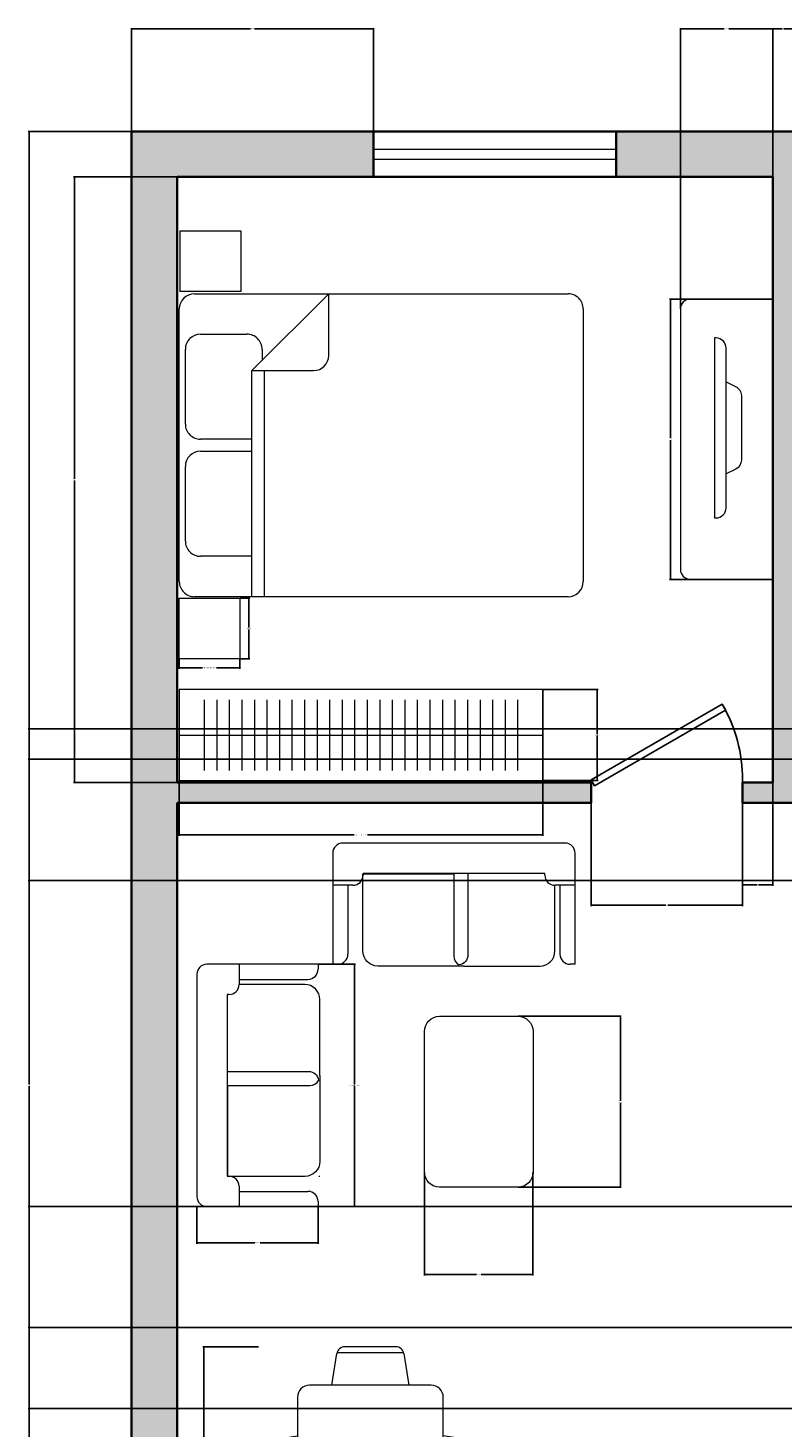
# Model space of a CAD drawing. Units: inches. Extents: x 1984 to 2284, y 2002 to 2421.
# Tile 2 of 4: x 1984 to 2134, y 2144 to 2421. Entities that reach past the tile are written whole.
import ezdxf

# ---------------------------------------------------------------- set-up
doc = ezdxf.new("R2010")
doc.units = ezdxf.units.IN
for name, color, linetype, lineweight in [('A-ANNO-DIMS', 2, 'Continuous', 18), ('A-DOOR', 3, 'Continuous', 25), ('A-EQPM', 9, 'Continuous', 18), ('A-FLOR-CASE', 9, 'Continuous', 20), ('A-FURN', 8, 'Continuous', 18), ('A-GLAZ', 4, 'Continuous', 18), ('A-WALL', 7, 'Continuous', 35)]:
    doc.layers.add(name, color=color, linetype=linetype, lineweight=lineweight)
doc.layers.add('A-WALL-PATT', color=18, linetype='Continuous', lineweight=13, true_color=0x000000)
doc.styles.get("Standard").update_dxf_attribs({"font": 'arial.ttf'})
doc.dimstyles.get("Standard").update_dxf_attribs({"dimtxt": 0.18, "dimasz": 0.18, "dimexe": 0.18, "dimexo": 0.0625, "dimgap": 0.09, "dimtad": 0, "dimtih": 1, "dimtoh": 1, "dimdec": 4, "dimzin": 0, "dimdsep": 46, "dimtxsty": 'Standard', "dimcen": 0.09, "dimadec": 0, "dimazin": 0, "dimtfac": 1, "dimtdec": 4, "dimtofl": 0, "dimtmove": 0, "dimatfit": 3, "dimfxl": 1, "dimtolj": 1, "dimtzin": 0, "dimarcsym": 0})

# ---------------------------------------------------------------- blocks, each defined once
blk = doc.blocks.new('Dining Set - 36 x 72 in.')
for p, q in [((-22.26, 25.81), (-23.48, 18)), ((-22.23, 26), (-5.76, 26)), ((-20.29, 27.5), (-7.71, 27.5)), ((-4.52, 18), (-5.74, 25.81)), ((5.74, 25.81), (4.52, 18)), ((5.77, 26), (22.24, 26)), ((7.71, 27.5), (20.29, 27.5)), ((23.48, 18), (22.26, 25.81)), ((33, 18), (-33, 18)), ((-36, 15), (-36, -15)), ((36, -15), (36, 15)), ((-44, 8.23), (-44, -8.24)), ((-43.81, 8.26), (-36, 9.48)), ((43.81, 8.26), (36, 9.48)), ((44, 8.23), (44, -8.24)), ((-45.5, 6.29), (-45.5, -6.29)), ((45.5, 6.29), (45.5, -6.29)), ((-36, -9.48), (-43.81, -8.26)), ((36, -9.48), (43.81, -8.26)), ((-33, -18), (33, -18)), ((-22.26, -25.81), (-23.48, -18)), ((-4.52, -18), (-5.74, -25.81)), ((5.74, -25.81), (4.52, -18)), ((23.48, -18), (22.26, -25.81)), ((-22.23, -26), (-5.76, -26)), ((-20.29, -27.5), (-7.71, -27.5)), ((5.77, -26), (22.24, -26)), ((7.71, -27.5), (20.29, -27.5))]:
    blk.add_line(p, q)
for centre, radius, start, end in [((-20.29, 25.5), 2, 90, 171.1198), ((-7.71, 25.5), 2, 8.881, 90), ((7.71, 25.5), 2, 90, 171.1198), ((20.29, 25.5), 2, 8.881, 90), ((-33, 15), 3, 90, 180), ((33, 15), 3, 0, 90), ((-43.5, 6.29), 2, 98.8806, 180), ((43.5, 6.29), 2, 0, 81.1194), ((-43.5, -6.29), 2, 180, 261.1194), ((43.5, -6.29), 2, 278.8806, 0), ((-33, -15), 3, 180, 270), ((33, -15), 3, 270, 0), ((-20.29, -25.5), 2, 188.8802, 270), ((-7.71, -25.5), 2, 270, 351.1191), ((7.71, -25.5), 2, 188.8802, 270), ((20.29, -25.5), 2, 270, 351.1191)]:
    blk.add_arc(centre, radius, start, end)
blk = doc.blocks.new('Bed - Queen')
for p, q in [((3, 0), (56.99999, 0)), ((10.99999, -1.2), (25.79998, -1.2)), ((34.19999, -1.2), (48.99999, -1.2)), ((0, -77.00003), (0, -3)), ((7.99999, -14.4), (7.99999, -4.2)), ((28.79998, -4.2), (28.79998, -14.4)), ((31.19999, -14.4), (31.19999, -4.2)), ((51.99999, -4.2), (51.99999, -13.4)), ((59.99999, -3), (59.99999, -77.00003)), ((0, -14.4), (44.8, -14.4)), ((59.99999, -29.6), (44.8, -14.4)), ((44.8, -14.4), (44.8, -26.6)), ((48.99999, -16.4), (46.79936, -16.4)), ((44.8, -16.8), (0, -16.8)), ((47.8, -29.6), (59.99999, -29.6)), ((56.99999, -80.00003), (3, -80.00003))]:
    blk.add_line(p, q)
for centre, start, end in [((3, -3), 90, 180), ((56.99999, -3), 0, 90), ((10.99999, -4.2), 90, 180), ((25.79998, -4.2), 0, 90), ((34.19999, -4.2), 90, 180), ((48.99999, -4.2), 0, 90), ((48.99999, -13.4), 270, 0), ((47.8, -26.6), 180, 270), ((3, -77.00003), 180, 270), ((56.99999, -77.00003), 270, 0)]:
    blk.add_arc(centre, 3, start, end)
blk = doc.blocks.new('*U10')
for p, q in [((0, 0), (0, -6)), ((40, 0), (40, -6))]:
    blk.add_line(p, q)
blk.add_lwpolyline([(0, 0), (34.64, 20), (35.52, 18.48), (0.87, -1.52)], close=True)
blk.add_arc((0, 0), 40, 0, 30)
blk = doc.blocks.new('GLAZING-48IN')
for p, q in [((0, 2), (48, 2)), ((0, 0), (48, 0))]:
    blk.add_line(p, q)
blk = doc.blocks.new('WARDROBE-72IN')
for p, q in [((72, 18), (0, 18)), ((0, 18), (0, 0)), ((4.97, 16), (4.97, 2)), ((7.45, 16), (7.45, 2)), ((9.93, 16), (9.93, 2)), ((12.41, 16), (12.41, 2)), ((14.9, 16), (14.9, 2)), ((17.38, 16), (17.38, 2)), ((19.86, 16), (19.86, 2)), ((22.34, 16), (22.34, 2)), ((24.83, 16), (24.83, 2)), ((27.31, 16), (27.31, 2)), ((29.79, 16), (29.79, 2)), ((32.28, 16), (32.28, 2)), ((34.76, 16), (34.76, 2)), ((37.24, 16), (37.24, 2)), ((39.72, 16), (39.72, 2)), ((42.21, 16), (42.21, 2)), ((44.69, 16), (44.69, 2)), ((47.17, 16), (47.17, 2)), ((49.66, 16), (49.66, 2)), ((52.14, 16), (52.14, 2)), ((54.62, 16), (54.62, 2)), ((57.1, 16), (57.1, 2)), ((59.59, 16), (59.59, 2)), ((62.07, 16), (62.07, 2)), ((64.55, 16), (64.55, 2)), ((67.03, 16), (67.03, 2)), ((0, 9), (72, 9)), ((0, 0), (72, 0))]:
    blk.add_line(p, q)
blk.add_lwpolyline([(72, 18), (72, 0)], close=True)
blk = doc.blocks.new('NIGHTSTAND-12IN')
blk.add_lwpolyline([(0, 12), (12, 12), (12, 0), (0, 0)], close=True)
blk = doc.blocks.new('LOVESEAT-FRAME-48IN')
for p, q in [((24, 48), (2, 48)), ((8.36, 48), (8.36, 44)), ((24, 48), (24, 47)), ((0, 46), (0, 2)), ((8.36, 45), (22, 45)), ((6, 42), (6, 6)), ((6.36, 42), (6, 42)), ((6, 6), (6.36, 6)), ((8.36, 4), (8.36, 0)), ((8.36, 3), (22, 3)), ((2, 0), (24, 0)), ((24, 1), (24, 0))]:
    blk.add_line(p, q)
for centre, start, end in [((2, 46), 90, 180), ((22, 47), 270, 0), ((6.36, 44), 270, 0), ((6.36, 4), 0, 90), ((22, 1), 0, 90), ((2, 2), 180, 270)]:
    blk.add_arc(centre, 2, start, end)
blk = doc.blocks.new('*D23')
at = {"layer": 'A-ANNO-DIMS', "color": 0, "lineweight": -2, "transparency": 16777216}
for p, q in [((2014.33, 2296.34), (2014.33, 2294.43)), ((2014.51, 2294.61), (2018.96, 2294.61)), ((2026.15, 2294.61), (2021.71, 2294.61)), ((2026.33, 2296.34), (2026.33, 2294.43))]:
    blk.add_line(p, q, dxfattribs=at)
at = {"layer": 'A-ANNO-DIMS', "color": 0, "transparency": 16777216}
for points in [[(2014.51, 2294.64), (2014.51, 2294.58), (2014.33, 2294.61)], [(2026.15, 2294.64), (2026.15, 2294.58), (2026.33, 2294.61)]]:
    blk.add_solid(points, dxfattribs=at)
at = {"layer": 'Defpoints', "color": 0, "transparency": 16777216}
for p in [(2014.33, 2296.41), (2026.33, 2296.41), (2026.33, 2294.61)]:
    blk.add_point(p, dxfattribs=at)
at = {"layer": 'A-ANNO-DIMS', "color": 0, "transparency": 16777216, "insert": (2020.33, 2294.61), "char_height": 0.18, "attachment_point": 5}
blk.add_mtext('\\A1;NIGHTSTAND 12 TYP.', dxfattribs=at)
blk = doc.blocks.new('*D24')
at = {"layer": 'A-ANNO-DIMS', "color": 0, "lineweight": -2, "transparency": 16777216}
for p, q in [((2026.4, 2308.41), (2028.31, 2308.41)), ((2028.13, 2308.23), (2028.13, 2302.59)), ((2028.13, 2296.59), (2028.13, 2302.23)), ((2026.4, 2296.41), (2028.31, 2296.41))]:
    blk.add_line(p, q, dxfattribs=at)
at = {"layer": 'A-ANNO-DIMS', "color": 0, "transparency": 16777216}
for points in [[(2028.1, 2308.23), (2028.16, 2308.23), (2028.13, 2308.41)], [(2028.1, 2296.59), (2028.16, 2296.59), (2028.13, 2296.41)]]:
    blk.add_solid(points, dxfattribs=at)
at = {"layer": 'Defpoints', "color": 0, "transparency": 16777216}
for p in [(2026.33, 2308.41), (2028.13, 2308.41), (2026.33, 2296.41)]:
    blk.add_point(p, dxfattribs=at)
at = {"layer": 'A-ANNO-DIMS', "color": 0, "transparency": 16777216, "insert": (2028.13, 2302.41), "char_height": 0.18, "attachment_point": 5}
blk.add_mtext('\\A1;12 TYP.', dxfattribs=at)
blk = doc.blocks.new('*D25')
at = {"layer": 'A-ANNO-DIMS', "color": 0, "lineweight": -2, "transparency": 16777216}
for p, q in [((2014.3, 2272.25), (2014.3, 2261.33)), ((2086.3, 2272.25), (2086.3, 2261.33)), ((2014.48, 2261.51), (2049, 2261.51)), ((2086.12, 2261.51), (2051.61, 2261.51))]:
    blk.add_line(p, q, dxfattribs=at)
at = {"layer": 'A-ANNO-DIMS', "color": 0, "transparency": 16777216}
for points in [[(2014.48, 2261.54), (2014.48, 2261.48), (2014.3, 2261.51)], [(2086.12, 2261.54), (2086.12, 2261.48), (2086.3, 2261.51)]]:
    blk.add_solid(points, dxfattribs=at)
at = {"layer": 'Defpoints', "color": 0, "transparency": 16777216}
for p in [(2014.3, 2272.31), (2086.3, 2272.31), (2086.3, 2261.51)]:
    blk.add_point(p, dxfattribs=at)
at = {"layer": 'A-ANNO-DIMS', "color": 0, "transparency": 16777216, "insert": (2050.3, 2261.51), "char_height": 0.18, "attachment_point": 5}
blk.add_mtext('\\A1;WARDROBE 72 TYP.', dxfattribs=at)
blk = doc.blocks.new('*D26')
at = {"layer": 'A-ANNO-DIMS', "color": 0, "lineweight": -2, "transparency": 16777216}
for p, q in [((2086.37, 2290.31), (2097.28, 2290.31)), ((2097.1, 2290.13), (2097.1, 2281.49)), ((2097.1, 2272.49), (2097.1, 2281.13)), ((2086.37, 2272.31), (2097.28, 2272.31))]:
    blk.add_line(p, q, dxfattribs=at)
at = {"layer": 'A-ANNO-DIMS', "color": 0, "transparency": 16777216}
for points in [[(2097.07, 2290.13), (2097.13, 2290.13), (2097.1, 2290.31)], [(2097.07, 2272.49), (2097.13, 2272.49), (2097.1, 2272.31)]]:
    blk.add_solid(points, dxfattribs=at)
at = {"layer": 'Defpoints', "color": 0, "transparency": 16777216}
for p in [(2086.3, 2290.31), (2097.1, 2290.31), (2086.3, 2272.31)]:
    blk.add_point(p, dxfattribs=at)
at = {"layer": 'A-ANNO-DIMS', "color": 0, "transparency": 16777216, "insert": (2097.1, 2281.31), "char_height": 0.18, "attachment_point": 5}
blk.add_mtext('\\A1;18 TYP.', dxfattribs=at)
blk = doc.blocks.new('*D27')
at = {"layer": 'A-ANNO-DIMS', "color": 0, "lineweight": -2, "transparency": 16777216}
for p, q in [((2041.88, 2235.9), (2049.2, 2235.9)), ((2049.02, 2235.72), (2049.02, 2212.09)), ((2049.02, 2188.08), (2049.02, 2211.72)), ((2041.88, 2187.9), (2049.2, 2187.9))]:
    blk.add_line(p, q, dxfattribs=at)
at = {"layer": 'A-ANNO-DIMS', "color": 0, "transparency": 16777216}
for points in [[(2048.99, 2235.72), (2049.05, 2235.72), (2049.02, 2235.9)], [(2048.99, 2188.08), (2049.05, 2188.08), (2049.02, 2187.9)]]:
    blk.add_solid(points, dxfattribs=at)
at = {"layer": 'Defpoints', "color": 0, "transparency": 16777216}
for p in [(2041.82, 2235.9), (2049.02, 2235.9), (2041.82, 2187.9)]:
    blk.add_point(p, dxfattribs=at)
at = {"layer": 'A-ANNO-DIMS', "color": 0, "transparency": 16777216, "insert": (2049.02, 2211.9), "char_height": 0.18, "attachment_point": 5}
blk.add_mtext('\\A1;LOVESEAT 48 TYP.', dxfattribs=at)
blk = doc.blocks.new('*D28')
at = {"layer": 'A-ANNO-DIMS', "color": 0, "lineweight": -2, "transparency": 16777216}
for p, q in [((2017.82, 2187.84), (2017.82, 2180.52)), ((2041.82, 2187.84), (2041.82, 2180.52)), ((2018, 2180.7), (2029.29, 2180.7)), ((2041.64, 2180.7), (2030.35, 2180.7))]:
    blk.add_line(p, q, dxfattribs=at)
at = {"layer": 'A-ANNO-DIMS', "color": 0, "transparency": 16777216}
for points in [[(2018, 2180.73), (2018, 2180.67), (2017.82, 2180.7)], [(2041.64, 2180.73), (2041.64, 2180.67), (2041.82, 2180.7)]]:
    blk.add_solid(points, dxfattribs=at)
at = {"layer": 'Defpoints', "color": 0, "transparency": 16777216}
for p in [(2017.82, 2187.9), (2041.82, 2187.9), (2041.82, 2180.7)]:
    blk.add_point(p, dxfattribs=at)
at = {"layer": 'A-ANNO-DIMS', "color": 0, "transparency": 16777216, "insert": (2029.82, 2180.7), "char_height": 0.18, "attachment_point": 5}
blk.add_mtext('\\A1;24 TYP.', dxfattribs=at)
blk = doc.blocks.new('*D39')
at = {"layer": 'A-ANNO-DIMS', "color": 0, "lineweight": -2, "transparency": 16777216}
for p, q in [((2030.05, 2160.11), (2018.99, 2160.11)), ((2019.17, 2159.93), (2019.17, 2123.8)), ((2019.17, 2087.31), (2019.17, 2123.44)), ((2030.05, 2087.13), (2018.99, 2087.13))]:
    blk.add_line(p, q, dxfattribs=at)
at = {"layer": 'A-ANNO-DIMS', "color": 0, "transparency": 16777216}
for points in [[(2019.14, 2159.93), (2019.2, 2159.93), (2019.17, 2160.11)], [(2019.14, 2087.31), (2019.2, 2087.31), (2019.17, 2087.13)]]:
    blk.add_solid(points, dxfattribs=at)
at = {"layer": 'Defpoints', "color": 0, "transparency": 16777216}
for p in [(2030.12, 2160.11), (2019.17, 2087.13), (2030.12, 2087.13)]:
    blk.add_point(p, dxfattribs=at)
at = {"layer": 'A-ANNO-DIMS', "color": 0, "transparency": 16777216, "insert": (2019.17, 2123.62), "char_height": 0.18, "attachment_point": 5}
blk.add_mtext('\\A1;DINING SET 73', dxfattribs=at)
blk = doc.blocks.new('*D42')
at = {"layer": 'A-ANNO-DIMS', "color": 0, "lineweight": -2, "transparency": 16777216}
for p, q in [((2004.82, 2400.91), (1984.41, 2400.91)), ((1984.59, 2400.73), (1984.59, 2212.09)), ((1984.59, 2023.09), (1984.59, 2211.73)), ((2004.82, 2022.91), (1984.41, 2022.91))]:
    blk.add_line(p, q, dxfattribs=at)
at = {"layer": 'A-ANNO-DIMS', "color": 0, "transparency": 16777216}
for points in [[(1984.56, 2400.73), (1984.62, 2400.73), (1984.59, 2400.91)], [(1984.56, 2023.09), (1984.62, 2023.09), (1984.59, 2022.91)]]:
    blk.add_solid(points, dxfattribs=at)
at = {"layer": 'Defpoints', "color": 0, "transparency": 16777216}
for p in [(1984.59, 2400.91), (2004.89, 2400.91), (2004.89, 2022.91)]:
    blk.add_point(p, dxfattribs=at)
at = {"layer": 'A-ANNO-DIMS', "color": 0, "transparency": 16777216, "insert": (1984.59, 2211.91), "char_height": 0.18, "attachment_point": 5}
blk.add_mtext('\\A1;378', dxfattribs=at)
blk = doc.blocks.new('*D43')
at = {"layer": 'A-ANNO-DIMS', "color": 0, "lineweight": -2, "transparency": 16777216}
for p, q in [((2004.89, 2400.97), (2004.89, 2421.39)), ((2005.07, 2421.21), (2028.46, 2421.21)), ((2052.64, 2421.21), (2029.25, 2421.21)), ((2052.82, 2400.97), (2052.82, 2421.39))]:
    blk.add_line(p, q, dxfattribs=at)
at = {"layer": 'A-ANNO-DIMS', "color": 0, "transparency": 16777216}
for points in [[(2005.07, 2421.24), (2005.07, 2421.18), (2004.89, 2421.21)], [(2052.64, 2421.24), (2052.64, 2421.18), (2052.82, 2421.21)]]:
    blk.add_solid(points, dxfattribs=at)
at = {"layer": 'Defpoints', "color": 0, "transparency": 16777216}
for p in [(2052.82, 2421.21), (2004.89, 2400.91), (2052.82, 2400.91)]:
    blk.add_point(p, dxfattribs=at)
at = {"layer": 'A-ANNO-DIMS', "color": 0, "transparency": 16777216, "insert": (2028.85, 2421.21), "char_height": 0.18, "attachment_point": 5}
blk.add_mtext('\\A1;47.93', dxfattribs=at)
blk = doc.blocks.new('*D44')
at = {"layer": 'A-ANNO-DIMS', "color": 0, "lineweight": -2, "transparency": 16777216}
for p, q in [((2113.56, 2365.76), (2113.56, 2421.39)), ((2113.74, 2421.21), (2122.27, 2421.21)), ((2131.71, 2421.21), (2123.18, 2421.21)), ((2131.89, 2367.76), (2131.89, 2421.39))]:
    blk.add_line(p, q, dxfattribs=at)
at = {"layer": 'A-ANNO-DIMS', "color": 0, "transparency": 16777216}
for points in [[(2113.74, 2421.24), (2113.74, 2421.18), (2113.56, 2421.21)], [(2131.71, 2421.24), (2131.71, 2421.18), (2131.89, 2421.21)]]:
    blk.add_solid(points, dxfattribs=at)
at = {"layer": 'Defpoints', "color": 0, "transparency": 16777216}
for p in [(2131.89, 2421.21), (2131.89, 2367.69), (2113.56, 2365.69)]:
    blk.add_point(p, dxfattribs=at)
at = {"layer": 'A-ANNO-DIMS', "color": 0, "transparency": 16777216, "insert": (2122.72, 2421.21), "char_height": 0.18, "attachment_point": 5}
blk.add_mtext('\\A1;18.328', dxfattribs=at)
blk = doc.blocks.new('*D45')
at = {"layer": 'A-ANNO-DIMS', "color": 0, "lineweight": -2, "transparency": 16777216}
for p, q in [((2131.89, 2391.97), (2131.89, 2421.39)), ((2132.07, 2421.21), (2133.73, 2421.21)), ((2135.71, 2421.21), (2134.04, 2421.21)), ((2135.89, 2391.97), (2135.89, 2421.39))]:
    blk.add_line(p, q, dxfattribs=at)
at = {"layer": 'A-ANNO-DIMS', "color": 0, "transparency": 16777216}
for points in [[(2132.07, 2421.24), (2132.07, 2421.18), (2131.89, 2421.21)], [(2135.71, 2421.24), (2135.71, 2421.18), (2135.89, 2421.21)]]:
    blk.add_solid(points, dxfattribs=at)
at = {"layer": 'Defpoints', "color": 0, "transparency": 16777216}
for p in [(2135.89, 2421.21), (2131.89, 2391.91), (2135.89, 2391.91)]:
    blk.add_point(p, dxfattribs=at)
at = {"layer": 'A-ANNO-DIMS', "color": 0, "transparency": 16777216, "insert": (2133.89, 2421.21), "char_height": 0.18, "attachment_point": 5}
blk.add_mtext('\\A1;4', dxfattribs=at)
blk = doc.blocks.new('*D49')
at = {"layer": 'A-ANNO-DIMS', "color": 0, "lineweight": -2, "transparency": 16777216}
for p, q in [((2013.82, 2391.91), (1993.41, 2391.91)), ((1993.59, 2391.73), (1993.59, 2332.09)), ((1993.59, 2272.09), (1993.59, 2331.73)), ((2013.82, 2271.91), (1993.41, 2271.91))]:
    blk.add_line(p, q, dxfattribs=at)
at = {"layer": 'A-ANNO-DIMS', "color": 0, "transparency": 16777216}
for points in [[(1993.56, 2391.73), (1993.62, 2391.73), (1993.59, 2391.91)], [(1993.56, 2272.09), (1993.62, 2272.09), (1993.59, 2271.91)]]:
    blk.add_solid(points, dxfattribs=at)
at = {"layer": 'Defpoints', "color": 0, "transparency": 16777216}
for p in [(1993.59, 2391.91), (2013.89, 2391.91), (2013.89, 2271.91)]:
    blk.add_point(p, dxfattribs=at)
at = {"layer": 'A-ANNO-DIMS', "color": 0, "transparency": 16777216, "insert": (1993.59, 2331.91), "char_height": 0.18, "attachment_point": 5}
blk.add_mtext('\\A1;120', dxfattribs=at)
blk = doc.blocks.new('*D63')
at = {"layer": 'A-ANNO-DIMS', "color": 0, "lineweight": -2, "transparency": 16777216}
for p, q in [((2095.89, 2267.85), (2095.89, 2247.43)), ((2125.89, 2267.85), (2125.89, 2247.43)), ((2096.07, 2247.61), (2110.67, 2247.61)), ((2125.71, 2247.61), (2111.1, 2247.61))]:
    blk.add_line(p, q, dxfattribs=at)
at = {"layer": 'A-ANNO-DIMS', "color": 0, "transparency": 16777216}
for points in [[(2096.07, 2247.64), (2096.07, 2247.58), (2095.89, 2247.61)], [(2125.71, 2247.64), (2125.71, 2247.58), (2125.89, 2247.61)]]:
    blk.add_solid(points, dxfattribs=at)
at = {"layer": 'Defpoints', "color": 0, "transparency": 16777216}
for p in [(2095.89, 2267.91), (2125.89, 2267.91), (2095.89, 2247.61)]:
    blk.add_point(p, dxfattribs=at)
at = {"layer": 'A-ANNO-DIMS', "color": 0, "transparency": 16777216, "insert": (2110.89, 2247.61), "char_height": 0.18, "attachment_point": 5}
blk.add_mtext('\\A1;30', dxfattribs=at)
blk = doc.blocks.new('*D64')
at = {"layer": 'A-ANNO-DIMS', "color": 0, "lineweight": -2, "transparency": 16777216}
for p, q in [((2125.89, 2271.85), (2125.89, 2251.43)), ((2131.89, 2271.85), (2131.89, 2251.43)), ((2126.07, 2251.61), (2128.74, 2251.61)), ((2131.71, 2251.61), (2129.03, 2251.61))]:
    blk.add_line(p, q, dxfattribs=at)
at = {"layer": 'A-ANNO-DIMS', "color": 0, "transparency": 16777216}
for points in [[(2126.07, 2251.64), (2126.07, 2251.58), (2125.89, 2251.61)], [(2131.71, 2251.64), (2131.71, 2251.58), (2131.89, 2251.61)]]:
    blk.add_solid(points, dxfattribs=at)
at = {"layer": 'Defpoints', "color": 0, "transparency": 16777216}
for p in [(2125.89, 2271.91), (2131.89, 2271.91), (2125.89, 2251.61)]:
    blk.add_point(p, dxfattribs=at)
at = {"layer": 'A-ANNO-DIMS', "color": 0, "transparency": 16777216, "insert": (2128.89, 2251.61), "char_height": 0.18, "attachment_point": 5}
blk.add_mtext('\\A1;6', dxfattribs=at)
blk = doc.blocks.new('*D69')
at = {"layer": 'A-ANNO-DIMS', "color": 0, "lineweight": -2, "transparency": 16777216}
for p, q in [((2177.82, 2276.51), (1984.41, 2276.51)), ((1984.59, 2276.33), (1984.59, 2264.69)), ((1984.59, 2252.69), (1984.59, 2264.33)), ((2177.82, 2252.51), (1984.41, 2252.51))]:
    blk.add_line(p, q, dxfattribs=at)
at = {"layer": 'A-ANNO-DIMS', "color": 0, "transparency": 16777216}
for points in [[(1984.56, 2276.33), (1984.62, 2276.33), (1984.59, 2276.51)], [(1984.56, 2252.69), (1984.62, 2252.69), (1984.59, 2252.51)]]:
    blk.add_solid(points, dxfattribs=at)
at = {"layer": 'Defpoints', "color": 0, "transparency": 16777216}
for p in [(1984.59, 2276.51), (2177.89, 2276.51), (2177.89, 2252.51)]:
    blk.add_point(p, dxfattribs=at)
at = {"layer": 'A-ANNO-DIMS', "color": 0, "transparency": 16777216, "insert": (1984.59, 2264.51), "char_height": 0.18, "attachment_point": 5}
blk.add_mtext('\\A1;24', dxfattribs=at)
blk = doc.blocks.new('*D70')
at = {"layer": 'A-ANNO-DIMS', "color": 0, "lineweight": -2, "transparency": 16777216}
for p, q in [((2177.82, 2282.51), (1984.41, 2282.51)), ((1984.59, 2282.33), (1984.59, 2279.7)), ((1984.59, 2276.69), (1984.59, 2279.33)), ((2177.82, 2276.51), (1984.41, 2276.51))]:
    blk.add_line(p, q, dxfattribs=at)
at = {"layer": 'A-ANNO-DIMS', "color": 0, "transparency": 16777216}
for points in [[(1984.56, 2282.33), (1984.62, 2282.33), (1984.59, 2282.51)], [(1984.56, 2276.69), (1984.62, 2276.69), (1984.59, 2276.51)]]:
    blk.add_solid(points, dxfattribs=at)
at = {"layer": 'Defpoints', "color": 0, "transparency": 16777216}
for p in [(1984.59, 2282.51), (2177.89, 2282.51), (2177.89, 2276.51)]:
    blk.add_point(p, dxfattribs=at)
at = {"layer": 'A-ANNO-DIMS', "color": 0, "transparency": 16777216, "insert": (1984.59, 2279.51), "char_height": 0.18, "attachment_point": 5}
blk.add_mtext('\\A1;6', dxfattribs=at)
blk = doc.blocks.new('*D71')
at = {"layer": 'A-ANNO-DIMS', "color": 0, "lineweight": -2, "transparency": 16777216}
for p, q in [((2177.82, 2187.91), (1984.41, 2187.91)), ((1984.59, 2187.73), (1984.59, 2176.09)), ((1984.59, 2164.09), (1984.59, 2175.73)), ((2177.82, 2163.91), (1984.41, 2163.91))]:
    blk.add_line(p, q, dxfattribs=at)
at = {"layer": 'A-ANNO-DIMS', "color": 0, "transparency": 16777216}
for points in [[(1984.56, 2187.73), (1984.62, 2187.73), (1984.59, 2187.91)], [(1984.56, 2164.09), (1984.62, 2164.09), (1984.59, 2163.91)]]:
    blk.add_solid(points, dxfattribs=at)
at = {"layer": 'Defpoints', "color": 0, "transparency": 16777216}
for p in [(1984.59, 2187.91), (2177.89, 2187.91), (2177.89, 2163.91)]:
    blk.add_point(p, dxfattribs=at)
at = {"layer": 'A-ANNO-DIMS', "color": 0, "transparency": 16777216, "insert": (1984.59, 2175.91), "char_height": 0.18, "attachment_point": 5}
blk.add_mtext('\\A1;24', dxfattribs=at)
blk = doc.blocks.new('*D72')
at = {"layer": 'A-ANNO-DIMS', "color": 0, "lineweight": -2, "transparency": 16777216}
for p, q in [((2181.82, 2163.91), (1984.41, 2163.91)), ((1984.59, 2163.73), (1984.59, 2156.09)), ((1984.59, 2148.09), (1984.59, 2155.73)), ((2181.82, 2147.91), (1984.41, 2147.91))]:
    blk.add_line(p, q, dxfattribs=at)
at = {"layer": 'A-ANNO-DIMS', "color": 0, "transparency": 16777216}
for points in [[(1984.56, 2163.73), (1984.62, 2163.73), (1984.59, 2163.91)], [(1984.56, 2148.09), (1984.62, 2148.09), (1984.59, 2147.91)]]:
    blk.add_solid(points, dxfattribs=at)
at = {"layer": 'Defpoints', "color": 0, "transparency": 16777216}
for p in [(1984.59, 2163.91), (2181.89, 2163.91), (2181.89, 2147.91)]:
    blk.add_point(p, dxfattribs=at)
at = {"layer": 'A-ANNO-DIMS', "color": 0, "transparency": 16777216, "insert": (1984.59, 2155.91), "char_height": 0.18, "attachment_point": 5}
blk.add_mtext('\\A1;16', dxfattribs=at)
blk = doc.blocks.new('*D77')
at = {"layer": 'A-ANNO-DIMS', "color": 0, "lineweight": -2, "transparency": 16777216}
for p, q in [((2062.9, 2194.66), (2062.9, 2174.24)), ((2084.38, 2194.66), (2084.38, 2174.24)), ((2063.08, 2174.42), (2073.18, 2174.42)), ((2084.2, 2174.42), (2074.11, 2174.42))]:
    blk.add_line(p, q, dxfattribs=at)
at = {"layer": 'A-ANNO-DIMS', "color": 0, "transparency": 16777216}
for points in [[(2063.08, 2174.45), (2063.08, 2174.39), (2062.9, 2174.42)], [(2084.2, 2174.45), (2084.2, 2174.39), (2084.38, 2174.42)]]:
    blk.add_solid(points, dxfattribs=at)
at = {"layer": 'Defpoints', "color": 0, "transparency": 16777216}
for p in [(2062.9, 2194.72), (2084.38, 2194.72), (2062.9, 2174.42)]:
    blk.add_point(p, dxfattribs=at)
at = {"layer": 'A-ANNO-DIMS', "color": 0, "transparency": 16777216, "insert": (2073.64, 2174.42), "char_height": 0.18, "attachment_point": 5}
blk.add_mtext('\\A1;21.487', dxfattribs=at)
blk = doc.blocks.new('*D78')
at = {"layer": 'A-ANNO-DIMS', "color": 0, "lineweight": -2, "transparency": 16777216}
for p, q in [((2081.45, 2225.59), (2101.86, 2225.59)), ((2101.68, 2225.41), (2101.68, 2208.84)), ((2101.68, 2191.9), (2101.68, 2208.47)), ((2081.45, 2191.72), (2101.86, 2191.72))]:
    blk.add_line(p, q, dxfattribs=at)
at = {"layer": 'A-ANNO-DIMS', "color": 0, "transparency": 16777216}
for points in [[(2101.65, 2225.41), (2101.71, 2225.41), (2101.68, 2225.59)], [(2101.65, 2191.9), (2101.71, 2191.9), (2101.68, 2191.72)]]:
    blk.add_solid(points, dxfattribs=at)
at = {"layer": 'Defpoints', "color": 0, "transparency": 16777216}
for p in [(2081.38, 2225.59), (2081.38, 2191.72), (2101.68, 2191.72)]:
    blk.add_point(p, dxfattribs=at)
at = {"layer": 'A-ANNO-DIMS', "color": 0, "transparency": 16777216, "insert": (2101.68, 2208.65), "char_height": 0.18, "attachment_point": 5}
blk.add_mtext('\\A1;33.865', dxfattribs=at)
blk = doc.blocks.new('*D79')
at = {"layer": 'A-ANNO-DIMS', "color": 0, "lineweight": -2, "transparency": 16777216}
for p, q in [((2131.82, 2367.69), (2111.41, 2367.69)), ((2111.59, 2367.51), (2111.59, 2340.11)), ((2111.59, 2312.34), (2111.59, 2339.74)), ((2131.82, 2312.16), (2111.41, 2312.16))]:
    blk.add_line(p, q, dxfattribs=at)
at = {"layer": 'A-ANNO-DIMS', "color": 0, "transparency": 16777216}
for points in [[(2111.56, 2367.51), (2111.62, 2367.51), (2111.59, 2367.69)], [(2111.56, 2312.34), (2111.62, 2312.34), (2111.59, 2312.16)]]:
    blk.add_solid(points, dxfattribs=at)
at = {"layer": 'Defpoints', "color": 0, "transparency": 16777216}
for p in [(2111.59, 2367.69), (2131.89, 2367.69), (2131.89, 2312.16)]:
    blk.add_point(p, dxfattribs=at)
at = {"layer": 'A-ANNO-DIMS', "color": 0, "transparency": 16777216, "insert": (2111.59, 2339.93), "char_height": 0.18, "attachment_point": 5}
blk.add_mtext('\\A1;55.53', dxfattribs=at)

msp = doc.modelspace()

# ---------------------------------------------------------------- hatches: boundary and pattern name
at = {"layer": 'A-WALL-PATT'}
h = msp.add_hatch(color=256, dxfattribs=at)
h.dxf.hatch_style = 1
h.paths.add_polyline_path([(2052.8198, 2400.9122), (2004.8852, 2400.9122), (2004.8852, 2022.9122), (2019.8852, 2022.9122), (2019.8852, 2031.9122), (2013.8852, 2031.9122), (2013.8852, 2267.9122), (2095.8852, 2267.9122), (2095.8852, 2271.9122), (2013.8852, 2271.9122), (2013.8852, 2391.9122), (2052.8198, 2391.9122)])
h = msp.add_hatch(color=256, dxfattribs=at)
h.dxf.hatch_style = 1
h.paths.add_polyline_path([(2178.9401, 2400.9122), (2100.8198, 2400.9122), (2100.8198, 2391.9122), (2131.8852, 2391.9122), (2131.8852, 2271.9122), (2125.8852, 2271.9122), (2125.8852, 2267.9122), (2135.8852, 2267.9122), (2135.8852, 2271.9122), (2135.8852, 2282.5141), (2141.8852, 2282.5141), (2141.8852, 2286.5141), (2135.8852, 2286.5141), (2135.8852, 2391.9122), (2178.9401, 2391.9122)])

# ---------------------------------------------------------------- linework, layer by layer
at = {"layer": 'A-EQPM'}
msp.add_lwpolyline([(2120.6166, 2359.9853), (2120.2923, 2359.9853), (2120.2923, 2324.3217), (2120.6166, 2324.3217, 0.41421356), (2122.6166, 2326.3217), (2122.6166, 2357.9853, 0.41421356)], format="xyb", close=True, dxfattribs=at)
msp.add_lwpolyline([(2122.6166, 2333.0395), (2122.6166, 2351.2675)], dxfattribs=at)
msp.add_lwpolyline([(2122.6166, 2351.2675), (2124.4994, 2350.3769, -0.28997444), (2125.6442, 2348.5689), (2125.6442, 2335.7812, -0.2849939), (2124.5325, 2333.9894), (2122.6166, 2333.0395)], format="xyb", dxfattribs=at)
at = {"layer": 'A-FLOR-CASE'}
msp.add_lwpolyline([(2131.8852, 2367.6926), (2115.5576, 2367.6926, 0.41421356), (2113.5576, 2365.6926), (2113.5576, 2314.1589, 0.41421356), (2115.5576, 2312.1589), (2131.8852, 2312.1589)], format="xyb", close=True, dxfattribs=at)
at = {"layer": 'A-FURN'}
msp.add_line((2042.1781, 2193.8629), (2041.9425, 2193.8629), dxfattribs=at)
for points in [[(2070.6823, 2235.5451), (2053.6823, 2235.5451, -0.41421356), (2050.6823, 2238.5451), (2050.6823, 2253.7807), (2068.6823, 2253.7807), (2068.6823, 2237.5451, 0.27352208), (2069.7185, 2235.7927)], [(2071.4997, 2253.9032), (2071.4997, 2237.7807, -0.38246106), (2069.7185, 2235.7927, -0.38246106)], [(2070.6823, 2235.5451), (2085.7227, 2235.5451, 0.41421356), (2088.7227, 2238.5451), (2088.7227, 2251.5451)], [(2042.1781, 2213.8629), (2042.1781, 2228.9032, 0.41421356), (2039.1781, 2231.9032), (2026.1781, 2231.9032)], [(2023.82, 2214.6803), (2039.9425, 2214.6803, -0.38246106), (2041.9305, 2212.8991, -0.38246106)], [(2042.1781, 2213.8629), (2042.1781, 2196.8629, -0.41421356), (2039.1781, 2193.8629), (2023.9425, 2193.8629), (2023.9425, 2211.8629), (2040.1781, 2211.8629, 0.27352208), (2041.9305, 2212.8991)]]:
    msp.add_lwpolyline(points, format="xyb", dxfattribs=at)
msp.add_lwpolyline([(2065.8974, 2225.586), (2081.3844, 2225.586, -0.41421356), (2084.3844, 2222.586), (2084.3844, 2194.7205, -0.41421356), (2081.3844, 2191.7205), (2065.8974, 2191.7205, -0.41421356), (2062.8974, 2194.7205), (2062.8974, 2222.586, -0.41421356)], format="xyb", close=True, dxfattribs=at)
at = {"layer": 'A-WALL'}
for p, q in [((2013.8852, 2391.9122), (2131.8852, 2391.9122)), ((2013.8852, 2271.9122), (2013.8852, 2391.9122)), ((2131.8852, 2271.9122), (2131.8852, 2391.9122)), ((2013.8852, 2271.9122), (2095.8852, 2271.9122)), ((2095.8852, 2271.9122), (2095.8852, 2267.9122)), ((2125.8852, 2271.9122), (2125.8852, 2267.9122)), ((2125.8852, 2271.9122), (2131.8852, 2271.9122)), ((2013.8852, 2031.9122), (2013.8852, 2267.9122)), ((2013.8852, 2267.9122), (2095.8852, 2267.9122)), ((2125.8852, 2267.9122), (2135.8852, 2267.9122))]:
    msp.add_line(p, q, dxfattribs=at)
for points in [[(2019.8852, 2022.9122), (2004.8852, 2022.9122), (2004.8852, 2400.9122), (2262.8852, 2400.9122), (2262.8852, 2022.9122), (2055.8852, 2022.9122)], [(2052.8198, 2391.9122), (2052.8198, 2400.9122)], [(2100.8198, 2400.9122), (2100.8198, 2391.9122)]]:
    msp.add_lwpolyline(points, dxfattribs=at)

# ---------------------------------------------------------------- block references
at = {"layer": 'A-DOOR', "xscale": 0.75, "yscale": 0.75, "zscale": 0.75}
msp.add_blockref('*U10', (2095.8852, 2272.4122), dxfattribs=at)
at = {"layer": 'A-FLOR-CASE'}
msp.add_blockref('WARDROBE-72IN', (2014.3042, 2272.3092), dxfattribs=at)
at = {"layer": 'A-FURN'}
for name, p in [('NIGHTSTAND-12IN', (2014.5272, 2369.1758)), ('NIGHTSTAND-12IN', (2014.3335, 2296.4062)), ('LOVESEAT-FRAME-48IN', (2017.82, 2187.9032))]:
    msp.add_blockref(name, p, dxfattribs=at)
for name, p, rotation in [('Bed - Queen', (2014.3345, 2308.7253), 89.99999999999999), ('LOVESEAT-FRAME-48IN', (2044.7227, 2259.9032), 270.0000000000029)]:
    msp.add_blockref(name, p, dxfattribs=dict(at, rotation=rotation))
at = {"layer": 'A-FURN', "xscale": 0.8020426707360627, "yscale": 0.8020426707360627, "zscale": 0.8020426707360627, "rotation": 270}
msp.add_blockref('Dining Set - 36 x 72 in.', (2052.1712, 2123.6218), dxfattribs=at)
at = {"layer": 'A-GLAZ'}
msp.add_blockref('GLAZING-48IN', (2052.8198, 2395.4122), dxfattribs=at)

# ---------------------------------------------------------------- dimensions: what is measured, and where the dimension line sits
at = {"layer": 'A-ANNO-DIMS'}
for base, p1, p2, override, picture, middle in [((2052.8198, 2421.2122), (2004.8852, 2400.9122), (2052.8198, 2400.9122), {"dimdec": 2, "dimlfac": 1, "dimrnd": 0, "dimzin": 0, "dimdsep": 46, "dimlunit": 2}, '*D43', (2028.8525, 2421.2122)), ((2131.8852, 2421.2122), (2113.5576, 2365.6926), (2131.8852, 2367.6926), {"dimdec": 3, "dimlfac": 1, "dimrnd": 0, "dimzin": 0, "dimdsep": 46, "dimlunit": 2}, '*D44', (2122.7214, 2421.2122)), ((2135.8852, 2421.2122), (2131.8852, 2391.9122), (2135.8852, 2391.9122), {"dimdec": 0, "dimlfac": 1, "dimrnd": 0, "dimzin": 0, "dimdsep": 46, "dimlunit": 2}, '*D45', (2133.8852, 2421.2122))]:
    dim = msp.add_linear_dim(base=base, p1=p1, p2=p2, dimstyle='Standard', override=override, dxfattribs=at)
    dim.commit()
    dim.dimension.update_dxf_attribs({"geometry": picture, "text_midpoint": middle})
for base, p1, p2, angle, override, picture, middle in [((1984.5852, 2400.9122), (2004.8852, 2022.9122), (2004.8852, 2400.9122), 90, {"dimdec": 0, "dimlfac": 1, "dimrnd": 0, "dimzin": 0, "dimdsep": 46, "dimlunit": 2}, '*D42', (1984.5852, 2211.9122)), ((1993.5852, 2391.9122), (2013.8852, 2271.9122), (2013.8852, 2391.9122), 90, {"dimdec": 0, "dimlfac": 1, "dimrnd": 0, "dimzin": 0, "dimdsep": 46, "dimlunit": 2}, '*D49', (1993.5852, 2331.9122)), ((2111.5852, 2367.6926), (2131.8852, 2312.1589), (2131.8852, 2367.6926), 90, {"dimdec": 2, "dimlfac": 1, "dimrnd": 0, "dimzin": 0, "dimdsep": 46, "dimlunit": 2}, '*D79', (2111.5852, 2339.9257)), ((1984.5852, 2282.5141), (2177.8852, 2276.5141), (2177.8852, 2282.5141), 90, {"dimdec": 0, "dimlfac": 1, "dimrnd": 0, "dimzin": 0, "dimdsep": 46, "dimlunit": 2}, '*D70', (1984.5852, 2279.5141)), ((1984.5852, 2276.5141), (2177.8852, 2252.5141), (2177.8852, 2276.5141), 90, {"dimdec": 0, "dimlfac": 1, "dimrnd": 0, "dimzin": 0, "dimdsep": 46, "dimlunit": 2}, '*D69', (1984.5852, 2264.5141)), ((2125.8852, 2251.6122), (2131.8852, 2271.9122), (2125.8852, 2271.9122), 180, {"dimdec": 0, "dimlfac": 1, "dimrnd": 0, "dimzin": 0, "dimdsep": 46, "dimlunit": 2}, '*D64', (2128.8852, 2251.6122)), ((2095.8852, 2247.6122), (2125.8852, 2267.9122), (2095.8852, 2267.9122), 180, {"dimdec": 0, "dimlfac": 1, "dimrnd": 0, "dimzin": 0, "dimdsep": 46, "dimlunit": 2}, '*D63', (2110.8852, 2247.6122)), ((2101.68436, 2191.72048), (2081.38436, 2225.58595), (2081.38436, 2191.72048), 270, {"dimdec": 3, "dimlfac": 1, "dimrnd": 0, "dimzin": 0, "dimdsep": 46, "dimlunit": 2}, '*D78', (2101.68436, 2208.65321)), ((2062.8974, 2174.4205), (2084.3844, 2194.7205), (2062.8974, 2194.7205), 180, {"dimdec": 3, "dimlfac": 1, "dimrnd": 0, "dimzin": 0, "dimdsep": 46, "dimlunit": 2}, '*D77', (2073.6409, 2174.4205)), ((1984.5852, 2187.9122), (2177.8852, 2163.9122), (2177.8852, 2187.9122), 90, {"dimdec": 0, "dimlfac": 1, "dimrnd": 0, "dimzin": 0, "dimdsep": 46, "dimlunit": 2}, '*D71', (1984.5852, 2175.9122)), ((1984.5852, 2163.9122), (2181.8852, 2147.9122), (2181.8852, 2163.9122), 90, {"dimdec": 0, "dimlfac": 1, "dimrnd": 0, "dimzin": 0, "dimdsep": 46, "dimlunit": 2}, '*D72', (1984.5852, 2155.9122))]:
    dim = msp.add_linear_dim(base=base, p1=p1, p2=p2, angle=angle, dimstyle='Standard', override=override, dxfattribs=at)
    dim.commit()
    dim.dimension.update_dxf_attribs({"geometry": picture, "text_midpoint": middle})
for base, p1, p2, angle, text, picture, middle in [((2028.1335, 2308.4062), (2026.3335, 2296.4062), (2026.3335, 2308.4062), 90, '<> TYP.', '*D24', (2028.1335, 2302.4062)), ((2097.1042, 2290.3092), (2086.3042, 2272.3092), (2086.3042, 2290.3092), 90, '<> TYP.', '*D26', (2097.1042, 2281.3092)), ((2049.02, 2235.9032), (2041.82, 2187.9032), (2041.82, 2235.9032), 90, 'LOVESEAT <> TYP.', '*D27', (2049.02, 2211.9032)), ((2019.1672, 2087.1288), (2030.115, 2160.1147), (2030.115, 2087.1288), 270, 'DINING SET <>', '*D39', (2019.1672, 2123.6218))]:
    dim = msp.add_linear_dim(base=base, p1=p1, p2=p2, angle=angle, text=text, dimstyle='Standard', override={"dimdec": 0, "dimlfac": 1, "dimrnd": 0, "dimzin": 0, "dimdsep": 46, "dimlunit": 2}, dxfattribs=at)
    dim.commit()
    dim.dimension.update_dxf_attribs({"geometry": picture, "text_midpoint": middle})
for base, p1, p2, text, picture, middle in [((2026.3335, 2294.6062), (2014.3335, 2296.4062), (2026.3335, 2296.4062), 'NIGHTSTAND <> TYP.', '*D23', (2020.3335, 2294.6062)), ((2086.3042, 2261.5092), (2014.3042, 2272.3092), (2086.3042, 2272.3092), 'WARDROBE <> TYP.', '*D25', (2050.3042, 2261.5092)), ((2041.82, 2180.7032), (2017.82, 2187.9032), (2041.82, 2187.9032), '<> TYP.', '*D28', (2029.82, 2180.7032))]:
    dim = msp.add_linear_dim(base=base, p1=p1, p2=p2, text=text, dimstyle='Standard', override={"dimdec": 0, "dimlfac": 1, "dimrnd": 0, "dimzin": 0, "dimdsep": 46, "dimlunit": 2}, dxfattribs=at)
    dim.commit()
    dim.dimension.update_dxf_attribs({"geometry": picture, "text_midpoint": middle})

doc.saveas('drawing.dxf')
